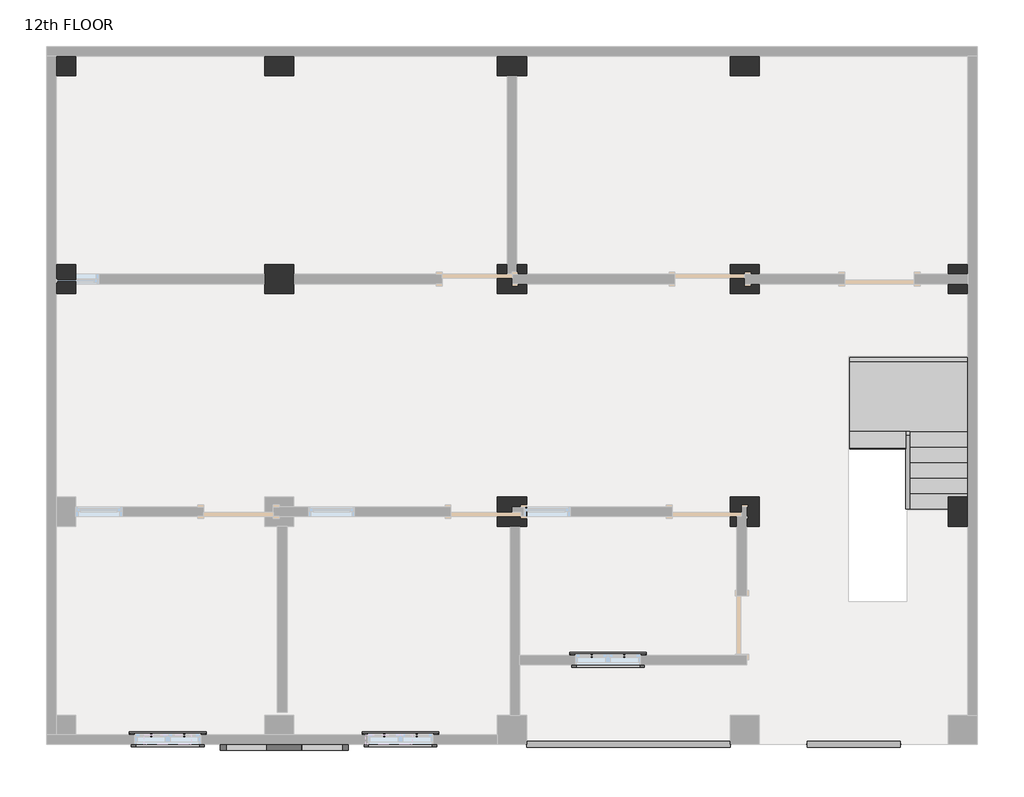
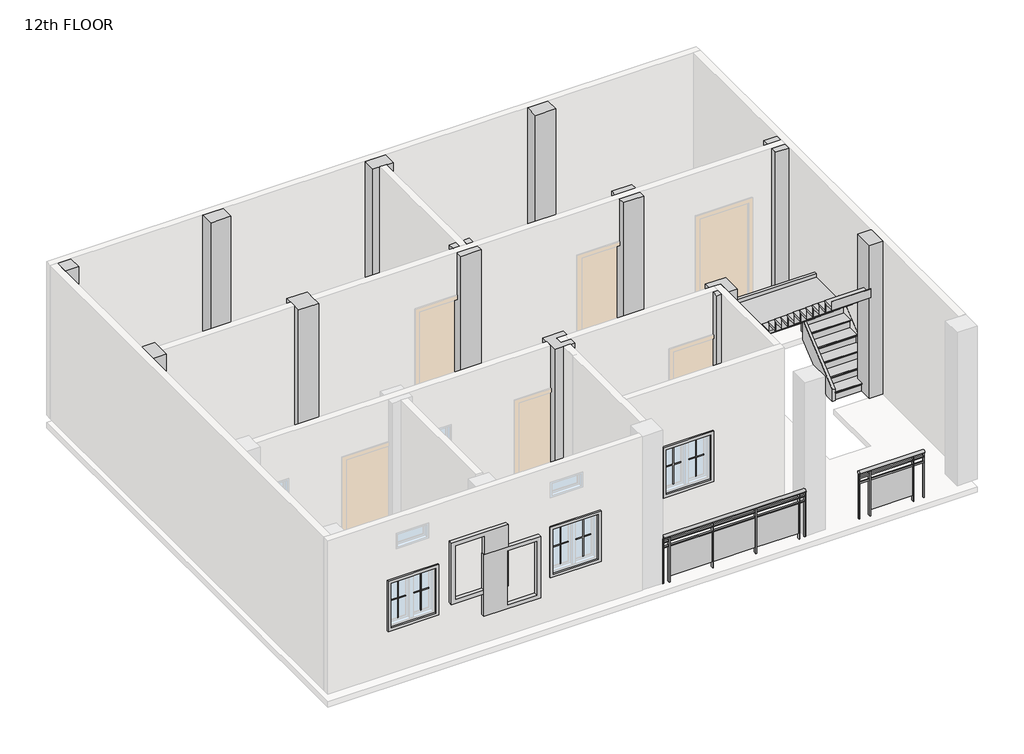
# One storey, part 2 of 2: 12 columns, 12 proxies, 4 members, 2 railings, 1 damper, 1 stair flight.
"""IFC4 building model written with IfcOpenShell, lengths in millimetres."""

from ifc_helpers import new_model, si_unit, point, frame, origin, place, context, project, spatial, polyline, ellipse_curve, trimmed, outline, extrude, faceted_brep, transform, mapped, element, save
from ifc_brep_helpers import plane_surface, extruded_surface, advanced_brep
from components import muntin_pattern_2x2_muntin_pattern_2x2_b3fe6957, muntin_pattern_2x2_muntin_pattern_2x2_3e0ecaf2, trim_window_exterior_flat_with_sill_41619996, trim_window_interior_flat_picture_frame_51c85655, duct_accessories_1_duct_accessories_1_838246fd, stair_flight_16fb6ac5

model = new_model("IFC4")

# Units and contexts
model_context = context("Model", 3, world=origin())
ifc_project = project(units=[si_unit("LENGTHUNIT", "METRE", prefix="MILLI")], contexts=[model_context])

# Site, building, storey
site = spatial("IfcSite", under=ifc_project)
building = spatial("IfcBuilding", under=site)
storey = spatial("IfcBuildingStorey", under=building, Name="12th FLOOR", Elevation=36423.6)

# Proxies
placement = place(None, origin())
muntin_pattern_2x2_muntin_pattern_2x2_shape = muntin_pattern_2x2_muntin_pattern_2x2_b3fe6957(model_context)
element("IfcBuildingElementProxy", 1, Name="Muntin Pattern_2x2 : Muntin Pattern_2x2", ObjectType="Muntin Pattern_2x2 : Muntin Pattern_2x2", at=placement, inside=storey, context=model_context, shape_type="MappedRepresentation", body=[
    mapped(muntin_pattern_2x2_muntin_pattern_2x2_shape, transform((-14441.409625, -253.8184478, 37407.85), x_axis=(1.0, 0.0, 0.0), y_axis=(0.0, 1.0, 0.0), z_axis=(0.0, 0.0, 1.0))),
])
element("IfcBuildingElementProxy", 2, Name="Muntin Pattern_2x2 : Muntin Pattern_2x2", ObjectType="Muntin Pattern_2x2 : Muntin Pattern_2x2", at=placement, inside=storey, context=model_context, shape_type="MappedRepresentation", body=[
    mapped(muntin_pattern_2x2_muntin_pattern_2x2_shape, transform((-11393.409625, -253.8184478, 37407.85), x_axis=(1.0, 0.0, 0.0), y_axis=(0.0, 1.0, 0.0), z_axis=(0.0, 0.0, 1.0))),
])
element("IfcBuildingElementProxy", 3, Name="Muntin Pattern_2x2 : Muntin Pattern_2x2", ObjectType="Muntin Pattern_2x2 : Muntin Pattern_2x2", at=placement, inside=storey, context=model_context, shape_type="MappedRepresentation", body=[
    mapped(muntin_pattern_2x2_muntin_pattern_2x2_shape, transform((-8675.609625, 787.5815522, 37407.85), x_axis=(1.0, 0.0, 0.0), y_axis=(0.0, 1.0, 0.0), z_axis=(0.0, 0.0, 1.0))),
])
muntin_pattern_2x2_muntin_pattern_2x2_2_shape = muntin_pattern_2x2_muntin_pattern_2x2_3e0ecaf2(model_context)
element("IfcBuildingElementProxy", 4, Name="Muntin Pattern_2x2 : Muntin Pattern_2x2", ObjectType="Muntin Pattern_2x2 : Muntin Pattern_2x2", at=placement, inside=storey, context=model_context, shape_type="MappedRepresentation", body=[
    mapped(muntin_pattern_2x2_muntin_pattern_2x2_2_shape, transform((-14012.784625, -253.8184478, 37407.85), x_axis=(-1.0, 0.0, 0.0), y_axis=(0.0, -1.0, 0.0), z_axis=(0.0, 0.0, 1.0))),
])
element("IfcBuildingElementProxy", 5, Name="Muntin Pattern_2x2 : Muntin Pattern_2x2", ObjectType="Muntin Pattern_2x2 : Muntin Pattern_2x2", at=placement, inside=storey, context=model_context, shape_type="MappedRepresentation", body=[
    mapped(muntin_pattern_2x2_muntin_pattern_2x2_2_shape, transform((-10964.784625, -253.8184478, 37407.85), x_axis=(-1.0, 0.0, 0.0), y_axis=(0.0, -1.0, 0.0), z_axis=(0.0, 0.0, 1.0))),
])
element("IfcBuildingElementProxy", 6, Name="Muntin Pattern_2x2 : Muntin Pattern_2x2", ObjectType="Muntin Pattern_2x2 : Muntin Pattern_2x2", at=placement, inside=storey, context=model_context, shape_type="MappedRepresentation", body=[
    mapped(muntin_pattern_2x2_muntin_pattern_2x2_2_shape, transform((-8246.984625, 787.5815522, 37407.85), x_axis=(-1.0, 0.0, 0.0), y_axis=(0.0, -1.0, 0.0), z_axis=(0.0, 0.0, 1.0))),
])
trim_window_exterior_flat_with_sill_shape = trim_window_exterior_flat_with_sill_41619996(model_context)
element("IfcBuildingElementProxy", 7, Name="Trim-Window-Exterior-Flat : with Sill", ObjectType="Trim-Window-Exterior-Flat : with Sill", at=placement, inside=storey, context=model_context, shape_type="MappedRepresentation", body=[
    mapped(trim_window_exterior_flat_with_sill_shape, transform((-14227.097125, -244.2934478, 38252.4), x_axis=(-1.0, 0.0, 0.0), y_axis=(0.0, 0.0, 1.0), z_axis=(0.0, 1.0, 0.0))),
])
element("IfcBuildingElementProxy", 8, Name="Trim-Window-Exterior-Flat : with Sill", ObjectType="Trim-Window-Exterior-Flat : with Sill", at=placement, inside=storey, context=model_context, shape_type="MappedRepresentation", body=[
    mapped(trim_window_exterior_flat_with_sill_shape, transform((-11179.097125, -244.2934478, 38252.4), x_axis=(-1.0, 0.0, 0.0), y_axis=(0.0, 0.0, 1.0), z_axis=(0.0, 1.0, 0.0))),
])
element("IfcBuildingElementProxy", 9, Name="Trim-Window-Exterior-Flat : with Sill", ObjectType="Trim-Window-Exterior-Flat : with Sill", at=placement, inside=storey, context=model_context, shape_type="MappedRepresentation", body=[
    mapped(trim_window_exterior_flat_with_sill_shape, transform((-8461.297125, 797.1065522, 38252.4), x_axis=(-1.0, 0.0, 0.0), y_axis=(0.0, 0.0, 1.0), z_axis=(0.0, 1.0, 0.0))),
])
trim_window_interior_flat_picture_frame_shape = trim_window_interior_flat_picture_frame_51c85655(model_context)
element("IfcBuildingElementProxy", 10, Name="Trim-Window-Interior-Flat : Picture Frame", ObjectType="Trim-Window-Interior-Flat : Picture Frame", at=placement, inside=storey, context=model_context, shape_type="MappedRepresentation", body=[
    mapped(trim_window_interior_flat_picture_frame_shape, transform((-14227.097125, -371.2934478, 38252.4), x_axis=(1.0, 0.0, 0.0), y_axis=(0.0, 0.0, 1.0), z_axis=(0.0, -1.0, 0.0))),
])
element("IfcBuildingElementProxy", 11, Name="Trim-Window-Interior-Flat : Picture Frame", ObjectType="Trim-Window-Interior-Flat : Picture Frame", at=placement, inside=storey, context=model_context, shape_type="MappedRepresentation", body=[
    mapped(trim_window_interior_flat_picture_frame_shape, transform((-11179.097125, -371.2934478, 38252.4), x_axis=(1.0, 0.0, 0.0), y_axis=(0.0, 0.0, 1.0), z_axis=(0.0, -1.0, 0.0))),
])
element("IfcBuildingElementProxy", 12, Name="Trim-Window-Interior-Flat : Picture Frame", ObjectType="Trim-Window-Interior-Flat : Picture Frame", at=placement, inside=storey, context=model_context, shape_type="MappedRepresentation", body=[
    mapped(trim_window_interior_flat_picture_frame_shape, transform((-8461.297125, 670.1065522, 38252.4), x_axis=(1.0, 0.0, 0.0), y_axis=(0.0, 0.0, 1.0), z_axis=(0.0, -1.0, 0.0))),
])

# Columns
element("IfcColumn", 13, ObjectType="column family : column family", at=placement, inside=storey, context=model_context, shape_type="SweptSolid", body=[
    extrude(outline(polyline([(-15433.597125, 8645.7065522), (-15433.597125, 8391.7065522), (-15687.597125, 8391.7065522), (-15687.597125, 8645.7065522), (-15433.597125, 8645.7065522)])), frame((0.0, 0.0, 36428.6), z_axis=(0.0, 0.0, 1.0), x_axis=(1.0, 0.0, 0.0)), (0.0, 0.0, 1.0), 3038.0),
])
element("IfcColumn", 14, ObjectType="column family : column family", at=placement, inside=storey, context=model_context, shape_type="SweptSolid", body=[
    extrude(outline(polyline([(-12576.097125, 5915.2065522), (-12576.097125, 5534.2065522), (-12957.097125, 5534.2065522), (-12957.097125, 5915.2065522), (-12576.097125, 5915.2065522)])), frame((0.0, 0.0, 36428.6), z_axis=(0.0, 0.0, 1.0), x_axis=(1.0, 0.0, 0.0)), (0.0, 0.0, 1.0), 3038.0),
])
element("IfcColumn", 15, ObjectType="column family : column family", at=placement, inside=storey, context=model_context, shape_type="Brep", body=[
    faceted_brep([(-9655.097125, 5915.2065522, 36428.6), (-9528.097125, 5915.2065522, 36428.6), (-9528.097125, 5788.2065522, 36428.6), (-9655.097125, 5788.2065522, 36428.6), (-9528.097125, 5915.2065522, 39466.6), (-9655.097125, 5915.2065522, 39466.6), (-9655.097125, 5788.2065522, 39466.6), (-9528.097125, 5788.2065522, 39466.6)], [[[0, 1, 2, 3]], [[4, 5, 6, 7]], [[0, 3, 6, 5]], [[4, 1, 0, 5]], [[3, 2, 7, 6]], [[1, 4, 7, 2]]]),
    faceted_brep([(-9528.097125, 5534.2065522, 39466.6), (-9528.097125, 5534.2065522, 36428.6), (-9528.097125, 5661.2065522, 36428.6), (-9528.097125, 5661.2065522, 39466.6), (-9909.097125, 5534.2065522, 36428.6), (-9909.097125, 5534.2065522, 39466.6), (-9909.097125, 5915.2065522, 36428.6), (-9909.097125, 5661.2065522, 39466.6), (-9909.097125, 5661.2065522, 38557.2), (-9909.097125, 5788.2065522, 38557.2), (-9909.097125, 5788.2065522, 39466.6), (-9909.097125, 5915.2065522, 39466.6), (-9782.097125, 5915.2065522, 39466.6), (-9782.097125, 5915.2065522, 36428.6), (-9782.097125, 5788.2065522, 36428.6), (-9782.097125, 5788.2065522, 39466.6), (-9782.097125, 5788.2065522, 38557.2), (-9718.597125, 5788.2065522, 36428.6), (-9718.597125, 5788.2065522, 38557.2), (-9718.597125, 5661.2065522, 36428.6), (-9718.597125, 5661.2065522, 38557.2)], [[[0, 1, 2, 3]], [[4, 1, 0, 5]], [[6, 4, 5, 7, 8, 9, 10, 11]], [[6, 11, 12, 13]], [[14, 13, 12, 15, 16]], [[17, 14, 16, 18]], [[19, 20, 8, 7, 3, 2]], [[1, 4, 6, 13, 14, 17, 19, 2]], [[5, 0, 3, 7]], [[12, 11, 10, 15]], [[9, 16, 15, 10]], [[18, 20, 19, 17]], [[20, 18, 16, 9, 8]]]),
])
element("IfcColumn", 16, ObjectType="column family : column family", at=placement, inside=storey, context=model_context, shape_type="Brep", body=[
    faceted_brep([(-6480.097125, 5534.2065522, 36428.6), (-6861.097125, 5534.2065522, 36428.6), (-6861.097125, 5915.2065522, 36428.6), (-6480.097125, 5915.2065522, 36428.6), (-6480.097125, 5788.2065522, 36428.6), (-6670.597125, 5788.2065522, 36428.6), (-6670.597125, 5661.2065522, 36428.6), (-6480.097125, 5661.2065522, 36428.6), (-6480.097125, 5534.2065522, 39466.6), (-6480.097125, 5661.2065522, 39466.6), (-6861.097125, 5534.2065522, 39466.6), (-6861.097125, 5661.2065522, 39466.6), (-6861.097125, 5661.2065522, 38557.2), (-6861.097125, 5788.2065522, 38557.2), (-6861.097125, 5788.2065522, 39466.6), (-6861.097125, 5915.2065522, 39466.6), (-6480.097125, 5915.2065522, 39466.6), (-6670.597125, 5661.2065522, 38557.2), (-6670.597125, 5788.2065522, 38557.2), (-6480.097125, 5788.2065522, 39466.6)], [[[0, 1, 2, 3, 4, 5, 6, 7]], [[8, 0, 7, 9]], [[1, 0, 8, 10]], [[2, 1, 10, 11, 12, 13, 14, 15]], [[3, 2, 15, 16]], [[10, 8, 9, 11]], [[6, 17, 12, 11, 9, 7]], [[13, 18, 5, 4, 19, 14]], [[3, 16, 19, 4]], [[16, 15, 14, 19]], [[18, 17, 6, 5]], [[17, 18, 13, 12]]]),
])
element("IfcColumn", 17, ObjectType="column family : column family", at=placement, inside=storey, context=model_context, shape_type="Brep", body=[
    faceted_brep([(-6480.097125, 2867.2065522, 36428.6), (-6480.097125, 2486.2065522, 36428.6), (-6645.197125, 2486.2065522, 36428.6), (-6645.197125, 2740.2065522, 36428.6), (-6708.697125, 2740.2065522, 36428.6), (-6708.697125, 2613.2065522, 36428.6), (-6772.197125, 2613.2065522, 36428.6), (-6772.197125, 2486.2065522, 36428.6), (-6861.097125, 2486.2065522, 36428.6), (-6861.097125, 2867.2065522, 36428.6), (-6480.097125, 2867.2065522, 39466.6), (-6480.097125, 2486.2065522, 39466.6), (-6861.097125, 2486.2065522, 39466.6), (-6772.197125, 2486.2065522, 39466.6), (-6861.097125, 2613.2065522, 39466.6), (-6861.097125, 2613.2065522, 38557.2), (-6861.097125, 2740.2065522, 38557.2), (-6861.097125, 2740.2065522, 39466.6), (-6861.097125, 2867.2065522, 39466.6), (-6772.197125, 2740.2065522, 39466.6), (-6645.197125, 2740.2065522, 39466.6), (-6645.197125, 2486.2065522, 39466.6), (-6772.197125, 2613.2065522, 39466.6), (-6772.197125, 2613.2065522, 38557.2), (-6772.197125, 2740.2065522, 38557.2), (-6708.697125, 2613.2065522, 38557.2), (-6708.697125, 2740.2065522, 38557.2)], [[[0, 1, 2, 3, 4, 5, 6, 7, 8, 9]], [[1, 0, 10, 11]], [[12, 8, 7, 13]], [[9, 8, 12, 14, 15, 16, 17, 18]], [[0, 9, 18, 10]], [[11, 10, 18, 17, 19, 20, 21]], [[15, 14, 22, 23]], [[17, 16, 24, 19]], [[20, 3, 2, 21]], [[6, 23, 22, 13, 7]], [[14, 12, 13, 22]], [[1, 11, 21, 2]], [[15, 23, 24, 16]], [[25, 23, 6, 5]], [[23, 25, 26, 24]], [[26, 25, 5, 4]], [[24, 26, 4, 3, 20, 19]]]),
])
element("IfcColumn", 18, ObjectType="column family : column family", at=placement, inside=storey, context=model_context, shape_type="Brep", body=[
    faceted_brep([(-9528.097125, 2486.2065522, 36428.6), (-9909.097125, 2486.2065522, 36428.6), (-9909.097125, 2867.2065522, 36428.6), (-9528.097125, 2867.2065522, 36428.6), (-9528.097125, 2740.2065522, 36428.6), (-9566.197125, 2740.2065522, 36428.6), (-9718.597125, 2740.2065522, 36428.6), (-9718.597125, 2613.2065522, 36428.6), (-9566.197125, 2613.2065522, 36428.6), (-9528.097125, 2613.2065522, 36428.6), (-9528.097125, 2486.2065522, 39466.6), (-9528.097125, 2613.2065522, 36728.4), (-9528.097125, 2740.2065522, 36728.4), (-9528.097125, 2867.2065522, 39466.6), (-9528.097125, 2740.2065522, 39466.6), (-9528.097125, 2740.2065522, 38557.2), (-9528.097125, 2613.2065522, 38557.2), (-9528.097125, 2613.2065522, 39466.6), (-9909.097125, 2486.2065522, 39466.6), (-9909.097125, 2867.2065522, 39466.6), (-9566.197125, 2613.2065522, 39466.6), (-9718.597125, 2613.2065522, 39466.6), (-9718.597125, 2740.2065522, 39466.6), (-9566.197125, 2740.2065522, 39466.6), (-9566.197125, 2613.2065522, 38557.2), (-9566.197125, 2613.2065522, 36728.4), (-9566.197125, 2740.2065522, 36728.4), (-9566.197125, 2740.2065522, 38557.2)], [[[0, 1, 2, 3, 4, 5, 6, 7, 8, 9]], [[10, 0, 9, 11, 12, 4, 3, 13, 14, 15, 16, 17]], [[1, 0, 10, 18]], [[2, 1, 18, 19]], [[3, 2, 19, 13]], [[18, 10, 17, 20, 21, 22, 23, 14, 13, 19]], [[11, 9, 8, 7, 21, 20, 17, 16, 24, 25]], [[4, 12, 26, 27, 15, 14, 23, 22, 6, 5]], [[21, 7, 6, 22]], [[25, 24, 27, 26]], [[25, 26, 12, 11]], [[27, 24, 16, 15]]]),
])
element("IfcColumn", 19, ObjectType="column family : column family", at=placement, inside=storey, context=model_context, shape_type="SweptSolid", body=[
    extrude(outline(polyline([(-12576.097125, 8391.7065522), (-12957.097125, 8391.7065522), (-12957.097125, 8645.7065522), (-12576.097125, 8645.7065522), (-12576.097125, 8391.7065522)])), frame((0.0, 0.0, 36428.6), z_axis=(0.0, 0.0, 1.0), x_axis=(1.0, 0.0, 0.0)), (0.0, 0.0, 1.0), 3038.0),
])
element("IfcColumn", 20, ObjectType="column family : column family", at=placement, inside=storey, context=model_context, shape_type="SweptSolid", body=[
    extrude(outline(polyline([(-9528.097125, 8391.7065522), (-9909.097125, 8391.7065522), (-9909.097125, 8645.7065522), (-9528.097125, 8645.7065522), (-9528.097125, 8391.7065522)])), frame((0.0, 0.0, 36428.6), z_axis=(0.0, 0.0, 1.0), x_axis=(1.0, 0.0, 0.0)), (0.0, 0.0, 1.0), 3038.0),
])
element("IfcColumn", 21, ObjectType="column family : column family", at=placement, inside=storey, context=model_context, shape_type="SweptSolid", body=[
    extrude(outline(polyline([(-6480.097125, 8391.7065522), (-6861.097125, 8391.7065522), (-6861.097125, 8645.7065522), (-6480.097125, 8645.7065522), (-6480.097125, 8391.7065522)])), frame((0.0, 0.0, 36428.6), z_axis=(0.0, 0.0, 1.0), x_axis=(1.0, 0.0, 0.0)), (0.0, 0.0, 1.0), 3038.0),
])
element("IfcColumn", 22, ObjectType="column family : column family", at=placement, inside=storey, context=model_context, shape_type="SweptSolid", body=[
    extrude(outline(polyline([(-4003.597125, 5915.2065522), (-3749.597125, 5915.2065522), (-3749.597125, 5788.2065522), (-4003.597125, 5788.2065522), (-4003.597125, 5915.2065522)])), frame((0.0, 0.0, 36428.6), z_axis=(0.0, 0.0, 1.0), x_axis=(1.0, 0.0, 0.0)), (0.0, 0.0, 1.0), 3038.0),
    extrude(outline(polyline([(-3749.597125, 5534.2065522), (-4003.597125, 5534.2065522), (-4003.597125, 5661.2065522), (-3749.597125, 5661.2065522), (-3749.597125, 5534.2065522)])), frame((0.0, 0.0, 36428.6), z_axis=(0.0, 0.0, 1.0), x_axis=(1.0, 0.0, 0.0)), (0.0, 0.0, 1.0), 3038.0),
])
element("IfcColumn", 23, ObjectType="column family : column family", at=placement, inside=storey, context=model_context, shape_type="SweptSolid", body=[
    extrude(outline(polyline([(-4003.597125, 2486.2065522), (-4003.597125, 2867.2065522), (-3749.597125, 2867.2065522), (-3749.597125, 2486.2065522), (-4003.597125, 2486.2065522)])), frame((0.0, 0.0, 36428.6), z_axis=(0.0, 0.0, 1.0), x_axis=(1.0, 0.0, 0.0)), (0.0, 0.0, 1.0), 3038.0),
])
element("IfcColumn", 24, ObjectType="column family : column family", at=placement, inside=storey, context=model_context, shape_type="SweptSolid", body=[
    extrude(outline(polyline([(-15433.597125, 5915.2065522), (-15433.597125, 5534.2065522), (-15687.597125, 5534.2065522), (-15687.597125, 5915.2065522), (-15433.597125, 5915.2065522)])), frame((0.0, 0.0, 36428.6), z_axis=(0.0, 0.0, 1.0), x_axis=(1.0, 0.0, 0.0)), (0.0, 0.0, 1.0), 3038.0),
])

# Damper
duct_accessories_1_duct_accessories_1_shape = duct_accessories_1_duct_accessories_1_838246fd(model_context)
element("IfcDamper", 25, ObjectType="Duct Accessories 1 : Duct Accessories 1", at=placement, inside=storey, context=model_context, shape_type="MappedRepresentation", body=[
    mapped(duct_accessories_1_duct_accessories_1_shape, transform((0.0, 0.0, 0.0), x_axis=(1.0, 0.0, 0.0), y_axis=(0.0, 1.0, 0.0), z_axis=(0.0, 0.0, 1.0))),
])

# Members
element("IfcMember", 26, ObjectType="Stringer - 2\" Width", at=placement, inside=storey, context=model_context, shape_type="SweptSolid", body=[
    extrude(outline(polyline([(2714.6319226, 36423.6), (2714.6319226, 36660.4438745), (3679.8319226, 37464.7772078), (3679.8319226, 37068.0165243), (2906.5320935, 36423.6), (2714.6319226, 36423.6)])), frame((-4563.0136682, 0.0, 0.0), z_axis=(1.0, 0.0, 0.0), x_axis=(0.0, 1.0, 0.0)), (0.0, 0.0, 1.0), 50.8),
])
element("IfcMember", 27, ObjectType="Stringer - 2\" Width", at=placement, inside=storey, context=model_context, shape_type="SweptSolid", body=[
    extrude(outline(polyline([(-4512.2136682, 3730.6319226), (-4512.2136682, 3679.8319226), (-4563.0136682, 3679.8319226), (-4563.0136682, 3730.6319226), (-4512.2136682, 3730.6319226)])), frame((0.0, 0.0, 37211.0), z_axis=(0.0, 0.0, 1.0), x_axis=(1.0, 0.0, 0.0)), (0.0, 0.0, 1.0), 304.8),
])
element("IfcMember", 28, ObjectType="Stringer - 2\" Width", at=placement, inside=storey, context=model_context, shape_type="SweptSolid", body=[
    extrude(outline(polyline([(2714.6319226, 36423.6), (2714.6319226, 36660.4438745), (3741.0592732, 37515.8), (4217.1720935, 37515.8), (2906.5320935, 36423.6), (2714.6319226, 36423.6)])), frame((-3749.597125, 0.0, 0.0), z_axis=(1.0, 0.0, 0.0), x_axis=(0.0, 1.0, 0.0)), (0.0, 0.0, 1.0), 50.8),
])
element("IfcMember", 29, ObjectType="Stringer - 2\" Width", at=placement, inside=storey, context=model_context, shape_type="SweptSolid", body=[
    extrude(outline(polyline([(-3698.797125, 4695.8319226), (-3698.797125, 4645.0319226), (-5295.0246464, 4645.0319226), (-5295.0246464, 4695.8319226), (-3698.797125, 4695.8319226)])), frame((0.0, 0.0, 37211.0), z_axis=(0.0, 0.0, 1.0), x_axis=(1.0, 0.0, 0.0)), (0.0, 0.0, 1.0), 304.8),
])

# Railings
element("IfcRailing", 30, ObjectType="Glass Panel - Bottom Fill", at=placement, inside=storey, context=model_context, shape_type="SolidModel", body=[
    advanced_brep(
    [(-9528.097125, -333.1934478, 37338.0), (-9528.097125, -409.3934478, 37338.0), (-6861.097125, -333.1934478, 37338.0), (-6861.097125, -409.3934478, 37338.0)],
    [
        (0, 1, ellipse_curve(frame((-9528.097125, -371.2934478, 37338.0), z_axis=(-1.0, 0.0, 0.0), x_axis=(0.0, -1.0, 0.0)), 38.1, 28.575)),
        (1, 0, ellipse_curve(frame((-9528.097125, -371.2934478, 37338.0), z_axis=(-1.0, 0.0, 0.0), x_axis=(0.0, -1.0, 0.0)), 38.1, 28.575)),
        (2, 3, ellipse_curve(frame((-6861.097125, -371.2934478, 37338.0), z_axis=(1.0, 0.0, 0.0), x_axis=(0.0, -1.0, 0.0)), 38.1, 28.575)),
        (3, 2, ellipse_curve(frame((-6861.097125, -371.2934478, 37338.0), z_axis=(1.0, 0.0, 0.0), x_axis=(0.0, -1.0, 0.0)), 38.1, 28.575)),
        (0, 2),
        (3, 1),
    ],
    [
        plane_surface(frame((-9528.097125, -371.2934478, 37338.0), z_axis=(-1.0, 0.0, 0.0), x_axis=(0.0, 1.0, 0.0))),
        plane_surface(frame((-6861.097125, -371.2934478, 37338.0), z_axis=(1.0, 0.0, 0.0), x_axis=(0.0, 1.0, 0.0))),
        extruded_surface(trimmed(ellipse_curve(frame((-6861.097125, -371.2934478, 37338.0), z_axis=(-1.0, 0.0, 0.0), x_axis=(0.0, -1.0, 0.0)), 38.1, 28.575), [point((-6861.097125, -333.1934478, 37338.0))], [point((-6861.097125, -409.3934478, 37338.0))], True, "CARTESIAN"), (-2667.0, 0.0, 0.0), 2667.0),
        extruded_surface(trimmed(ellipse_curve(frame((-6861.097125, -371.2934478, 37338.0), z_axis=(-1.0, 0.0, 0.0), x_axis=(0.0, -1.0, 0.0)), 38.1, 28.575), [point((-6861.097125, -409.3934478, 37338.0))], [point((-6861.097125, -333.1934478, 37338.0))], True, "CARTESIAN"), (-2667.0, 0.0, 0.0), 2667.0),
    ],
    [
        (0, [[1, 2]]),
        (1, [[3, 4]]),
        (2, [[-1, 5, -4, 6]]),
        (3, [[-2, -6, -3, -5]]),
    ],
),
    extrude(outline(polyline([(-9528.097125, -383.9934478), (-9528.097125, -358.5934478), (-6861.097125, -358.5934478), (-6861.097125, -383.9934478), (-9528.097125, -383.9934478)])), frame((0.0, 0.0, 37223.7), z_axis=(0.0, 0.0, 1.0), x_axis=(1.0, 0.0, 0.0)), (0.0, 0.0, 1.0), 25.4),
    extrude(outline(polyline([(-9528.097125, -383.9934478), (-9528.097125, -358.5934478), (-6861.097125, -358.5934478), (-6861.097125, -383.9934478), (-9528.097125, -383.9934478)])), frame((0.0, 0.0, 37122.1), z_axis=(0.0, 0.0, 1.0), x_axis=(1.0, 0.0, 0.0)), (0.0, 0.0, 1.0), 25.4),
    extrude(outline(polyline([(-6981.747125, -396.6934478), (-6981.747125, -345.8934478), (-6969.047125, -345.8934478), (-6969.047125, -396.6934478), (-6981.747125, -396.6934478)])), frame((0.0, 0.0, 36423.6), z_axis=(0.0, 0.0, 1.0), x_axis=(1.0, 0.0, 0.0)), (0.0, 0.0, 1.0), 885.6788223),
    extrude(outline(polyline([(-7788.197125, -364.7582908), (-6975.397125, -364.7582908), (-6975.397125, -371.1082908), (-7788.197125, -371.1082908), (-7788.197125, -364.7582908)])), frame((0.0, 0.0, 36525.2), z_axis=(0.0, 0.0, 1.0), x_axis=(1.0, 0.0, 0.0)), (0.0, 0.0, 1.0), 596.9),
    extrude(outline(polyline([(-7794.547125, -396.6934478), (-7794.547125, -345.8934478), (-7781.847125, -345.8934478), (-7781.847125, -396.6934478), (-7794.547125, -396.6934478)])), frame((0.0, 0.0, 36423.6), z_axis=(0.0, 0.0, 1.0), x_axis=(1.0, 0.0, 0.0)), (0.0, 0.0, 1.0), 885.6788223),
    extrude(outline(polyline([(-8600.997125, -364.7582908), (-7788.197125, -364.7582908), (-7788.197125, -371.1082908), (-8600.997125, -371.1082908), (-8600.997125, -364.7582908)])), frame((0.0, 0.0, 36525.2), z_axis=(0.0, 0.0, 1.0), x_axis=(1.0, 0.0, 0.0)), (0.0, 0.0, 1.0), 596.9),
    extrude(outline(polyline([(-8607.347125, -396.6934478), (-8607.347125, -345.8934478), (-8594.647125, -345.8934478), (-8594.647125, -396.6934478), (-8607.347125, -396.6934478)])), frame((0.0, 0.0, 36423.6), z_axis=(0.0, 0.0, 1.0), x_axis=(1.0, 0.0, 0.0)), (0.0, 0.0, 1.0), 885.6788223),
    extrude(outline(polyline([(-9413.797125, -364.7582908), (-8600.997125, -364.7582908), (-8600.997125, -371.1082908), (-9413.797125, -371.1082908), (-9413.797125, -364.7582908)])), frame((0.0, 0.0, 36525.2), z_axis=(0.0, 0.0, 1.0), x_axis=(1.0, 0.0, 0.0)), (0.0, 0.0, 1.0), 596.9),
    extrude(outline(polyline([(-9420.147125, -396.6934478), (-9420.147125, -345.8934478), (-9407.447125, -345.8934478), (-9407.447125, -396.6934478), (-9420.147125, -396.6934478)])), frame((0.0, 0.0, 36423.6), z_axis=(0.0, 0.0, 1.0), x_axis=(1.0, 0.0, 0.0)), (0.0, 0.0, 1.0), 885.6788223),
    extrude(outline(polyline([(-6873.797125, -380.8184478), (-6873.797125, -361.7684478), (-6854.747125, -361.7684478), (-6854.747125, -380.8184478), (-6873.797125, -380.8184478)])), frame((0.0, 0.0, 36423.6), z_axis=(0.0, 0.0, 1.0), x_axis=(1.0, 0.0, 0.0)), (0.0, 0.0, 1.0), 885.6788223),
    extrude(outline(polyline([(-9534.447125, -380.8184478), (-9534.447125, -361.7684478), (-9515.397125, -361.7684478), (-9515.397125, -380.8184478), (-9534.447125, -380.8184478)])), frame((0.0, 0.0, 36423.6), z_axis=(0.0, 0.0, 1.0), x_axis=(1.0, 0.0, 0.0)), (0.0, 0.0, 1.0), 885.6788223),
])
element("IfcRailing", 31, ObjectType="Glass Panel - Bottom Fill", at=placement, inside=storey, context=model_context, shape_type="SolidModel", body=[
    advanced_brep(
    [(-5851.447125, -333.1934478, 37338.0), (-5851.447125, -409.3934478, 37338.0), (-4632.247125, -333.1934478, 37338.0), (-4632.247125, -409.3934478, 37338.0)],
    [
        (0, 1, ellipse_curve(frame((-5851.447125, -371.2934478, 37338.0), z_axis=(-1.0, 0.0, 0.0), x_axis=(0.0, -1.0, 0.0)), 38.1, 28.575)),
        (1, 0, ellipse_curve(frame((-5851.447125, -371.2934478, 37338.0), z_axis=(-1.0, 0.0, 0.0), x_axis=(0.0, -1.0, 0.0)), 38.1, 28.575)),
        (2, 3, ellipse_curve(frame((-4632.247125, -371.2934478, 37338.0), z_axis=(1.0, 0.0, 0.0), x_axis=(0.0, -1.0, 0.0)), 38.1, 28.575)),
        (3, 2, ellipse_curve(frame((-4632.247125, -371.2934478, 37338.0), z_axis=(1.0, 0.0, 0.0), x_axis=(0.0, -1.0, 0.0)), 38.1, 28.575)),
        (0, 2),
        (3, 1),
    ],
    [
        plane_surface(frame((-5851.447125, -371.2934478, 37338.0), z_axis=(-1.0, 0.0, 0.0), x_axis=(0.0, 1.0, 0.0))),
        plane_surface(frame((-4632.247125, -371.2934478, 37338.0), z_axis=(1.0, 0.0, 0.0), x_axis=(0.0, 1.0, 0.0))),
        extruded_surface(trimmed(ellipse_curve(frame((-4632.247125, -371.2934478, 37338.0), z_axis=(-1.0, 0.0, 0.0), x_axis=(0.0, -1.0, 0.0)), 38.1, 28.575), [point((-4632.247125, -333.1934478, 37338.0))], [point((-4632.247125, -409.3934478, 37338.0))], True, "CARTESIAN"), (-1219.1999999999998, 0.0, 0.0), 1219.1999999999998),
        extruded_surface(trimmed(ellipse_curve(frame((-4632.247125, -371.2934478, 37338.0), z_axis=(-1.0, 0.0, 0.0), x_axis=(0.0, -1.0, 0.0)), 38.1, 28.575), [point((-4632.247125, -409.3934478, 37338.0))], [point((-4632.247125, -333.1934478, 37338.0))], True, "CARTESIAN"), (-1219.1999999999998, 0.0, 0.0), 1219.1999999999998),
    ],
    [
        (0, [[1, 2]]),
        (1, [[3, 4]]),
        (2, [[-1, 5, -4, 6]]),
        (3, [[-2, -6, -3, -5]]),
    ],
),
    extrude(outline(polyline([(-5851.447125, -383.9934478), (-5851.447125, -358.5934478), (-4632.247125, -358.5934478), (-4632.247125, -383.9934478), (-5851.447125, -383.9934478)])), frame((0.0, 0.0, 37223.7), z_axis=(0.0, 0.0, 1.0), x_axis=(1.0, 0.0, 0.0)), (0.0, 0.0, 1.0), 25.4),
    extrude(outline(polyline([(-5851.447125, -383.9934478), (-5851.447125, -358.5934478), (-4632.247125, -358.5934478), (-4632.247125, -383.9934478), (-5851.447125, -383.9934478)])), frame((0.0, 0.0, 37122.1), z_axis=(0.0, 0.0, 1.0), x_axis=(1.0, 0.0, 0.0)), (0.0, 0.0, 1.0), 25.4),
    extrude(outline(polyline([(-4841.797125, -396.6934478), (-4841.797125, -345.8934478), (-4829.097125, -345.8934478), (-4829.097125, -396.6934478), (-4841.797125, -396.6934478)])), frame((0.0, 0.0, 36423.6), z_axis=(0.0, 0.0, 1.0), x_axis=(1.0, 0.0, 0.0)), (0.0, 0.0, 1.0), 885.6788223),
    extrude(outline(polyline([(-5648.247125, -364.7582908), (-4835.447125, -364.7582908), (-4835.447125, -371.1082908), (-5648.247125, -371.1082908), (-5648.247125, -364.7582908)])), frame((0.0, 0.0, 36525.2), z_axis=(0.0, 0.0, 1.0), x_axis=(1.0, 0.0, 0.0)), (0.0, 0.0, 1.0), 596.9),
    extrude(outline(polyline([(-5654.597125, -396.6934478), (-5654.597125, -345.8934478), (-5641.897125, -345.8934478), (-5641.897125, -396.6934478), (-5654.597125, -396.6934478)])), frame((0.0, 0.0, 36423.6), z_axis=(0.0, 0.0, 1.0), x_axis=(1.0, 0.0, 0.0)), (0.0, 0.0, 1.0), 885.6788223),
    extrude(outline(polyline([(-4644.947125, -380.8184478), (-4644.947125, -361.7684478), (-4625.897125, -361.7684478), (-4625.897125, -380.8184478), (-4644.947125, -380.8184478)])), frame((0.0, 0.0, 36423.6), z_axis=(0.0, 0.0, 1.0), x_axis=(1.0, 0.0, 0.0)), (0.0, 0.0, 1.0), 885.6788223),
    extrude(outline(polyline([(-5857.797125, -380.8184478), (-5857.797125, -361.7684478), (-5838.747125, -361.7684478), (-5838.747125, -380.8184478), (-5857.797125, -380.8184478)])), frame((0.0, 0.0, 36423.6), z_axis=(0.0, 0.0, 1.0), x_axis=(1.0, 0.0, 0.0)), (0.0, 0.0, 1.0), 885.6788223),
])

# Stair flight
stair_flight_shape = stair_flight_16fb6ac5(model_context)
element("IfcStairFlight", 32, ObjectType="2\" Tread 1\" Nosing 1/4\" Riser", at=placement, inside=storey, context=model_context, shape_type="MappedRepresentation", body=[
    mapped(stair_flight_shape, transform((0.0, 0.0, 0.0), x_axis=(1.0, 0.0, 0.0), y_axis=(0.0, 1.0, 0.0), z_axis=(0.0, 0.0, 1.0))),
])

save(model, "model.ifc")

# Revit data of these elements
# Type "Muntin Pattern_2x2 : Muntin Pattern_2x2"
#   Width [instance default] = 4' - 0"
#   Thickness = 0' - 0 1/2"
#   Height [instance default] = 4' - 0"
#   Distance = 0' - 0 3/4"
#   Interior Material [instance default] = none
#   Exterior Material [instance default] = none
#   Default Elevation = 0
# Type "Trim-Window-Exterior-Flat : with Sill"
#   Trim Width = 0' - 2 1/4"
#   Trim Thickness_Picture Frame = 0' - 1 1/4"
#   Trim Thickness_with Sill = 0' - 0 3/4"
#   Sill Thickness = 0' - 1 1/4"
#   Opening Width [instance default] = 2' - 0"
#   Opening Height [instance default] = 3' - 0"
#   Default Elevation = 4' - 0"
#   Sill = yes
#   Picture Frame = no
#   Trim Material [instance default] = none
# Type "Trim-Window-Interior-Flat : Picture Frame"
#   Trim Thickness_Picture Frame = 0' - 1 1/4"
#   Trim Width = 0' - 2 1/4"
#   Trim Thickness_with Sill = 0' - 0 3/4"
#   Sill Thickness = 0' - 1 1/4"
#   Opening Width [instance default] = 2' - 0"
#   Opening Height [instance default] = 3' - 0"
#   Default Elevation = 4' - 0"
#   Sill = no
#   Picture Frame = yes
#   Trim Material [instance default] = none
# Type "column family : column family"
#   w2 [instance default] = 0' - 9.88189"
#   w1 [instance default] = 0' - 9.01575"
#   Depth = 1' - 11.62205"
#   Width = 1' - 11.62205"
# Type "Glass Panel - Bottom Fill"
#   Assembly Code = "C2010400"
#   built-in parameter 1008612 = 0.0416667 (stored number, unit not read)
#   built-in parameter 1008611 = 0.0416667 (stored number, unit not read)
#   built-in parameter 1008609 = 0.333333 (stored number, unit not read)
#   built-in parameter 1008604 = 0.166667 (stored number, unit not read)
#   built-in parameter 1008603 = 0.166667 (stored number, unit not read)
#   Railing Height = 3' - 0"
#   built-in parameter 1008630 = 2
#   built-in parameter 1008610 = 2
#   built-in parameter 1008618 = Baluster - Square : 3/4"
# Elements 1, 2, 3, 4, 5, 6 (IfcBuildingElementProxy, "Muntin Pattern_2x2 : Muntin Pattern_2x2")
#   Width = 0' - 11 5/8"
#   Height = 2' - 6 1/2"
#   Interior Material = Wood - Stained
#   Exterior Material = Clad - White
#   Phase Created = New Construction
#   Materials on its faces: "Clad - White", "Wood - Stained"
# Elements 7, 8, 9 (IfcBuildingElementProxy, "Trim-Window-Exterior-Flat : with Sill")
#   Opening Width = 2' - 10"
#   Opening Height = 3' - 0"
#   Trim Material = Clad - White
#   Phase Created = New Construction
#   Materials on its faces: "Clad - White"
# Elements 10, 11, 12 (IfcBuildingElementProxy, "Trim-Window-Interior-Flat : Picture Frame")
#   Opening Width = 2' - 10"
#   Opening Height = 3' - 0"
#   Trim Material = Wood - Stained
#   Phase Created = New Construction
#   Materials on its faces: "Wood - Stained"
# Elements 13, 14, 15, 19, 20, 21 (IfcColumn, "column family : column family")
#   w2 = 1' - 3"
#   w1 = 1' - 3"
#   Phase Created = New Construction
#   Materials on its faces: "Default Wall"
# Elements 16, 22, 23 (IfcColumn, "column family : column family")
#   w2 = 1' - 3"
#   w1 = 1' - 3"
#   Phase Created = New Construction
#   Materials on its faces: "grey", "Default Wall"
# Element 17 (IfcColumn, "column family : column family")
#   w2 = 1' - 3"
#   w1 = 1' - 3"
#   Phase Created = New Construction
#   Materials on its faces: "Default Wall", "grey", "inside wall"
# Element 18 (IfcColumn, "column family : column family")
#   w2 = 1' - 3"
#   w1 = 1' - 3"
#   Phase Created = New Construction
#   Materials on its faces: "Default Wall", "inside wall"
# Element 24 (IfcColumn, "column family : column family")
#   w2 = 1' - 3"
#   w1 = 1' - 3"
#   Phase Created = New Construction
#   Materials on its faces: "inside wall", "Default Wall"
# Element 25 (IfcDamper, "Duct Accessories 1 : Duct Accessories 1")
#   Mark = "1"
#   Phase Created = New Construction
#   Materials on its faces: "border"
# Elements 26, 27, 28, 29 (IfcMember, "Stringer - 2\" Width")
#   Phase Created = New Construction
# Elements 30, 31 (IfcRailing, "Glass Panel - Bottom Fill")
#   Phase Created = New Construction
#   Materials on its faces: "Glass"
# Element 32 (IfcStairFlight, "2\" Tread 1\" Nosing 1/4\" Riser")
#   Phase Created = New Construction
# Materials
#   "Clad - White": class "Wood", colour RGB 242 242 238, transparency 0, Cost = 0
#   "Wood - Stained": class "Wood", colour RGB 224 178 126, transparency 0, Cost = 0
#   "Default Wall": colour RGB 128 128 128, transparency 0, Cost = 0
#   "grey": class "Generic", colour RGB 80 80 80, transparency 0, Cost = 0
#   "inside wall": class "Generic", colour RGB 199 224 95, transparency 0, Cost = 0
#   "border": class "Generic", colour RGB 144 144 144, transparency 0, Cost = 0
#   "Glass": class "Glass", colour RGB 0 128 192, transparency 0.75, Description = "Soda Lime Glass", Cost = 0
